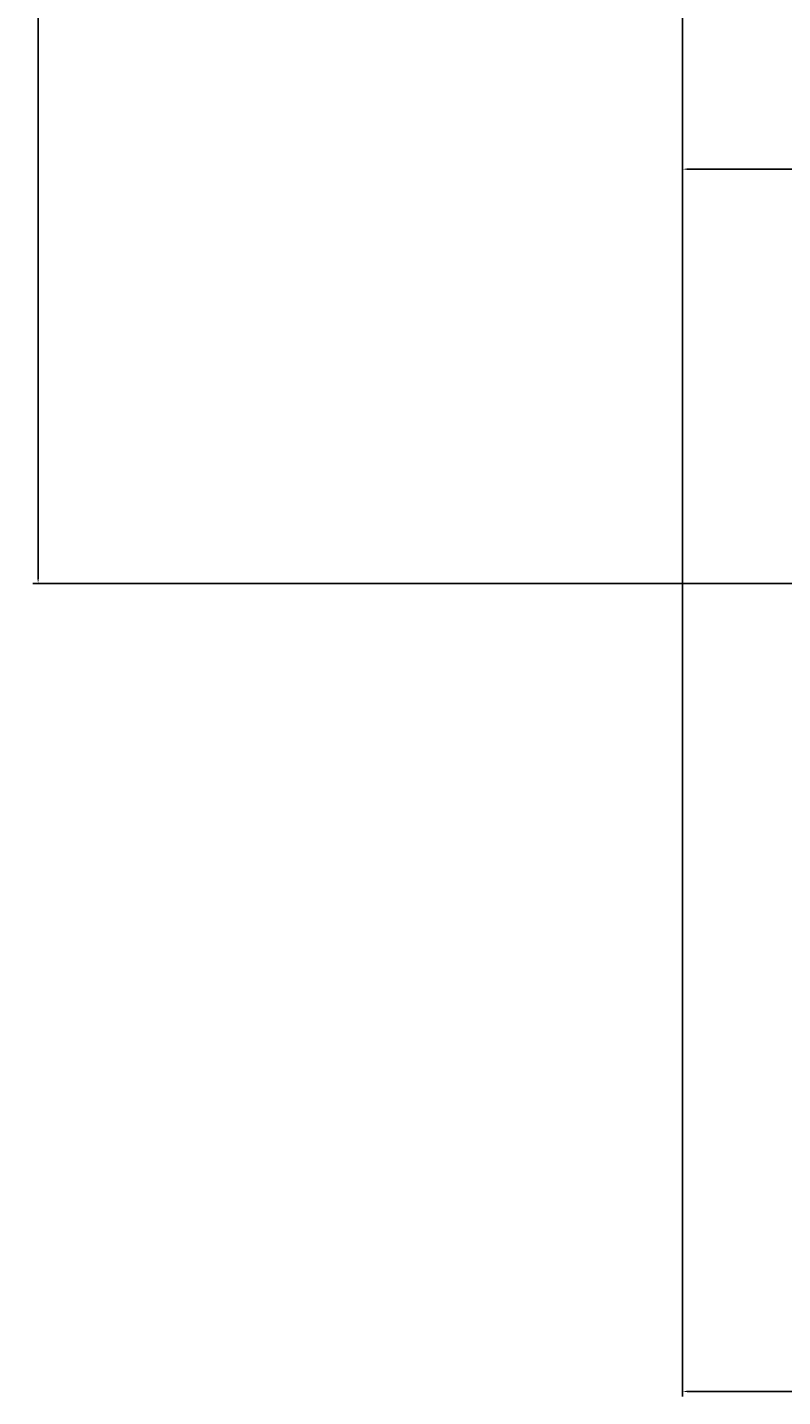
# Model space of a CAD drawing. Units: inches. Extents: x -1 to 292, y -3 to 199.
# Tile 1 of 52: x -1 to 25, y -3 to 45. Entities that reach past the tile are written whole.
import ezdxf

# ---------------------------------------------------------------- set-up
doc = ezdxf.new("R2010")
doc.units = ezdxf.units.IN
doc.header["$MEASUREMENT"] = 0
doc.layers.add('M-DIMS', color=2, linetype='Continuous', lineweight=18)
doc.styles.get("Standard").update_dxf_attribs({"font": 'arial.ttf'})
doc.dimstyles.get("Standard").update_dxf_attribs({"dimtxt": 0.18, "dimasz": 0.18, "dimexe": 0.18, "dimexo": 0.0625, "dimgap": 0.09, "dimtad": 0, "dimtih": 1, "dimtoh": 1, "dimdec": 4, "dimzin": 0, "dimdsep": 46, "dimtxsty": 'Standard', "dimcen": 0.09, "dimadec": 0, "dimazin": 0, "dimtfac": 1, "dimtdec": 4, "dimtofl": 0, "dimtmove": 0, "dimatfit": 3, "dimfxl": 1, "dimtolj": 1, "dimtzin": 0, "dimarcsym": 0})

# ---------------------------------------------------------------- blocks, each defined once
blk = doc.blocks.new('*D7')
at = {"layer": 'Defpoints', "color": 0, "transparency": 16777216}
for p in [(21.861, 54.582), (205.115, 54.582), (21.861, 39.982)]:
    blk.add_point(p, dxfattribs=at)
at = {"layer": 'M-DIMS', "color": 0, "lineweight": -2, "transparency": 16777216}
for p, q in [((21.861, 54.52), (21.861, 39.802)), ((205.115, 54.52), (205.115, 39.802)), ((22.041, 39.982), (113.033, 39.982)), ((204.935, 39.982), (113.944, 39.982))]:
    blk.add_line(p, q, dxfattribs=at)
at = {"layer": 'M-DIMS', "color": 0, "transparency": 16777216}
for points in [[(22.041, 40.012), (22.041, 39.952), (21.861, 39.982)], [(204.935, 40.012), (204.935, 39.952), (205.115, 39.982)]]:
    blk.add_solid(points, dxfattribs=at)
at = {"layer": 'M-DIMS', "color": 0, "transparency": 16777216, "insert": (113.488, 39.982), "char_height": 0.18, "attachment_point": 5}
blk.add_mtext('\\A1;183.25', dxfattribs=at)
blk = doc.blocks.new('*D8')
at = {"layer": 'Defpoints', "color": 0, "transparency": 16777216}
for p in [(-0.662, 126.765), (111.488, 126.765), (69.013, 25.514)]:
    blk.add_point(p, dxfattribs=at)
at = {"layer": 'M-DIMS', "color": 0, "lineweight": -2, "transparency": 16777216}
for p, q in [((111.426, 126.765), (-0.842, 126.765)), ((-0.662, 126.585), (-0.662, 76.321)), ((-0.662, 25.694), (-0.662, 75.958)), ((68.951, 25.514), (-0.842, 25.514))]:
    blk.add_line(p, q, dxfattribs=at)
at = {"layer": 'M-DIMS', "color": 0, "transparency": 16777216}
for points in [[(-0.692, 126.585), (-0.632, 126.585), (-0.662, 126.765)], [(-0.692, 25.694), (-0.632, 25.694), (-0.662, 25.514)]]:
    blk.add_solid(points, dxfattribs=at)
at = {"layer": 'M-DIMS', "color": 0, "transparency": 16777216, "insert": (-0.662, 76.14), "char_height": 0.18, "attachment_point": 5}
blk.add_mtext('\\A1;101.25', dxfattribs=at)
blk = doc.blocks.new('*D23')
at = {"layer": 'Defpoints', "color": 0, "transparency": 16777216}
for p in [(21.861, 54.582), (64.679, 51.267), (64.679, -2.71)]:
    blk.add_point(p, dxfattribs=at)
at = {"layer": 'M-DIMS', "color": 0, "lineweight": -2, "transparency": 16777216}
for p, q in [((21.861, 54.52), (21.861, -2.89)), ((64.679, 51.205), (64.679, -2.89)), ((22.041, -2.71), (42.874, -2.71)), ((64.499, -2.71), (43.666, -2.71))]:
    blk.add_line(p, q, dxfattribs=at)
at = {"layer": 'M-DIMS', "color": 0, "transparency": 16777216}
for points in [[(22.041, -2.68), (22.041, -2.74), (21.861, -2.71)], [(64.499, -2.68), (64.499, -2.74), (64.679, -2.71)]]:
    blk.add_solid(points, dxfattribs=at)
at = {"layer": 'M-DIMS', "color": 0, "transparency": 16777216, "insert": (43.27, -2.71), "char_height": 0.18, "attachment_point": 5}
blk.add_mtext('\\A1;42.82', dxfattribs=at)

msp = doc.modelspace()

# ---------------------------------------------------------------- dimensions: what is measured, and where the dimension line sits
at = {"layer": 'M-DIMS'}
for base, p1, p2, angle, picture, middle in [((-0.6625, 126.765), (69.013, 25.5141), (111.4883, 126.765), 90, '*D8', (-0.6625, 76.1396)), ((21.8612, 39.9821), (205.1155, 54.5821), (21.8612, 54.5821), 180, '*D7', (113.4883, 39.9821))]:
    dim = msp.add_linear_dim(base=base, p1=p1, p2=p2, angle=angle, dimstyle='Standard', override={"dimdec": 2, "dimlfac": 1, "dimrnd": 0, "dimzin": 0, "dimdsep": 46, "dimlunit": 2}, dxfattribs=at)
    dim.commit()
    dim.dimension.update_dxf_attribs({"geometry": picture, "text_midpoint": middle})
dim = msp.add_linear_dim(base=(64.6788, -2.7104), p1=(21.8612, 54.5821), p2=(64.6788, 51.2672), dimstyle='Standard', override={"dimdec": 2, "dimlfac": 1, "dimrnd": 0, "dimzin": 0, "dimdsep": 46, "dimlunit": 2}, dxfattribs=at)
dim.commit()
dim.dimension.update_dxf_attribs({"geometry": '*D23', "text_midpoint": (43.27, -2.7104)})

doc.saveas('drawing.dxf')
